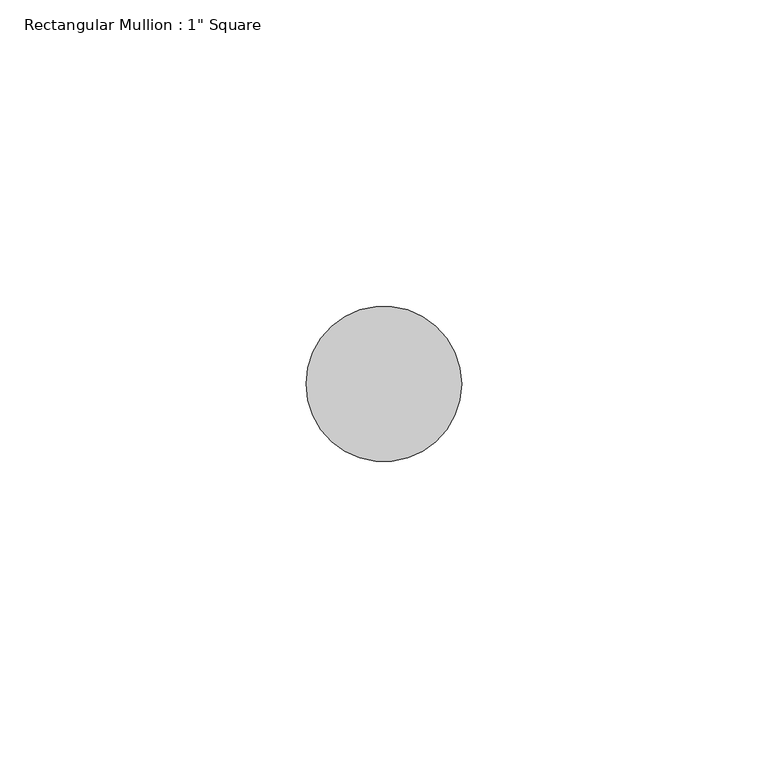
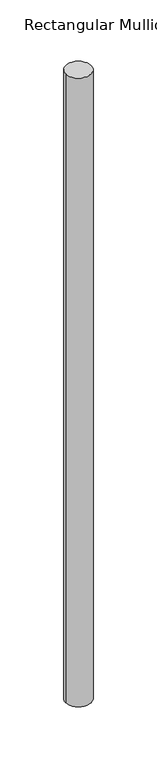
"""IFC4 building model written with IfcOpenShell, lengths in millimetres: member geometry."""

from ifc_helpers import new_model, si_unit, point, frame, origin, origin_2d, place, context, project, spatial, circle_curve, trimmed, segment, composite_curve, outline, extrude, source, transform, mapped, element, save


def member_6b6d42fb(model_context):
    return source(origin(), model_context, "Body", "SweptSolid", [
        extrude(outline(composite_curve([segment(trimmed(circle_curve(origin_2d(), 12.7), [point((12.7, 0.0))], [point((-12.7, 0.0))], False, "CARTESIAN"), True, "CONTINUOUS"), segment(trimmed(circle_curve(origin_2d(), 12.7), [point((-12.7, 0.0))], [point((12.7, 0.0))], False, "CARTESIAN"), True, "CONTINUOUS")], self_intersect=False)), frame((0.0, 0.0, -659.511), z_axis=(0.0, 0.0, 1.0), x_axis=(1.0, 0.0, 0.0)), (0.0, 0.0, 1.0), 659.511),
    ])


if __name__ == "__main__":
    model = new_model("IFC4")
    model_context = context("Model", 3, world=origin())
    ifc_project = project(units=[si_unit("LENGTHUNIT", "METRE", prefix="MILLI")], contexts=[model_context])
    site = spatial("IfcSite", under=ifc_project)
    building = spatial("IfcBuilding", under=site)
    placement = place(None, origin())
    member_shape = member_6b6d42fb(model_context)
    element("IfcMember", 1, ObjectType="Rectangular Mullion : 1\" Square", at=placement, inside=building, context=model_context, shape_type="MappedRepresentation", body=[
        mapped(member_shape, transform((0.0, 0.0, 0.0), x_axis=(1.0, 0.0, 0.0), y_axis=(0.0, 1.0, 0.0), z_axis=(0.0, 0.0, 1.0))),
    ])
    save(model, "model.ifc")

# Revit data of these elements
# Type "Rectangular Mullion : 1\" Square"
#   built-in parameter 1007350 = 0.0416667 (stored number, unit not read)
# Element 1 (IfcMember, "Rectangular Mullion : 1\" Square")
#   Materials on its faces: "Aluminum"
# Materials
#   "Aluminum": class "Metal", colour RGB 247 247 247, transparency 0, Description = "Aluminum 6061", Cost = 0
